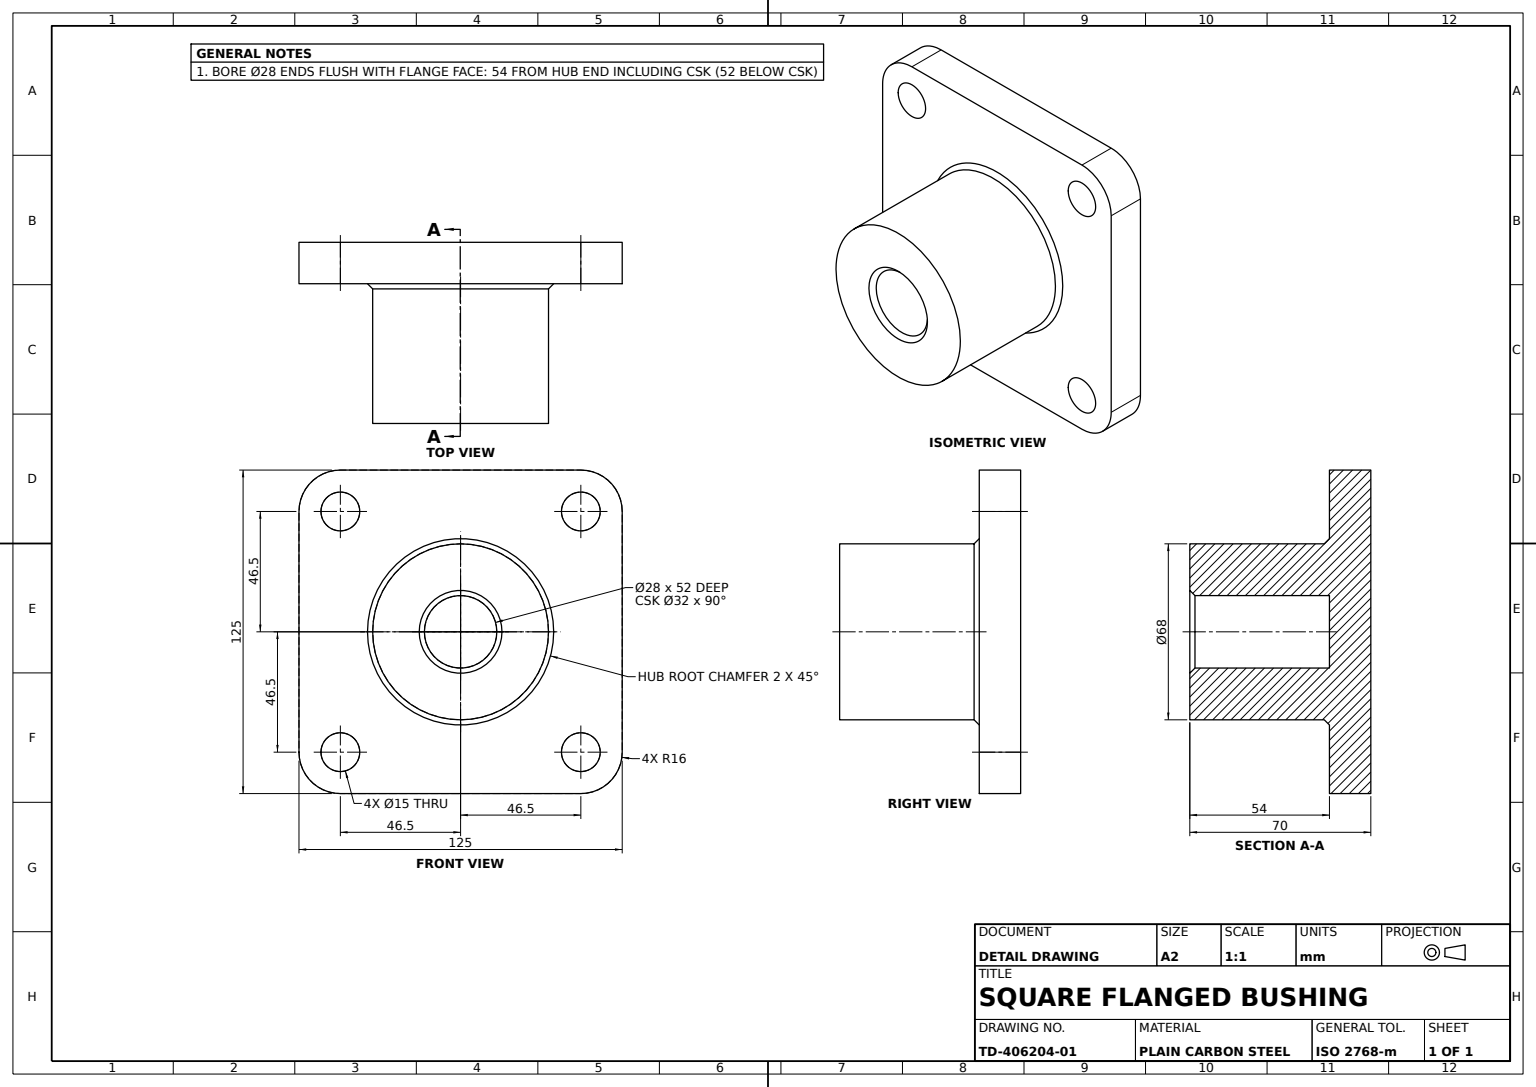
from build123d import *

# Parameters (mm, degrees)
FLANGE_PLATE_125X125X16_DEPTH = 16
BOLT_HOLES_SKETCH_R           = 7.5
BOLT_HOLES_4X_15_DEPTH        = 16
HUB_SKETCH_R                  = 34
HUB_68X54_DEPTH               = 54
HUB_CHAMFER_2X45_SIZE         = 2
BORE_SKETCH_R                 = 14
BORE_28_DEPTH                 = 54
BORE_CHAMFER_2X45_SIZE        = 2


with BuildPart() as part:
    # Flange Plate Sketch → Flange Plate 125x125x16 (new body)
    with BuildSketch(Plane.XY):
        with BuildLine():
            Line((16, 0), (109, 0))
            ThreePointArc((109, 0), (120.313708499, -4.686291501), (125, -16))
            Line((125, -16), (125, -109))
            ThreePointArc((125, -109), (120.313708499, -120.313708499), (109, -125))
            Line((109, -125), (16, -125))
            ThreePointArc((16, -125), (4.686291501, -120.313708499), (0, -109))
            Line((0, -109), (0, -16))
            ThreePointArc((0, -16), (4.686291501, -4.686291501), (16, 0))
        make_face()
    extrude(amount=FLANGE_PLATE_125X125X16_DEPTH)

    # Bolt Holes Sketch → Bolt Holes 4xØ15 (cut)
    with BuildSketch(Plane.XY.offset(16)):
        with Locations((16, -16)):
            Circle(BOLT_HOLES_SKETCH_R)
        with Locations((109, -16)):
            Circle(BOLT_HOLES_SKETCH_R)
        with Locations((109, -109)):
            Circle(BOLT_HOLES_SKETCH_R)
        with Locations((16, -109)):
            Circle(BOLT_HOLES_SKETCH_R)
    extrude(amount=-BOLT_HOLES_4X_15_DEPTH, mode=Mode.SUBTRACT)

    # Hub Sketch → Hub Ø68x54 (add)
    with BuildSketch(Plane.XY.offset(16)):
        with Locations((62.5, -62.5)):
            Circle(HUB_SKETCH_R)
    extrude(amount=HUB_68X54_DEPTH)

    # Hub Chamfer 2x45
    hub_chamfer_2x45_edges = [part.edges().sort_by_distance(p)[0] for p in [
        (28.5, -62.5, 16),
    ]]
    chamfer(hub_chamfer_2x45_edges, length=HUB_CHAMFER_2X45_SIZE)

    # Bore Sketch → Bore Ø28 (cut)
    with BuildSketch(Plane.XY.offset(70)):
        with Locations((62.5, -62.5)):
            Circle(BORE_SKETCH_R)
    extrude(amount=-BORE_28_DEPTH, mode=Mode.SUBTRACT)

    # Bore Chamfer 2x45
    bore_chamfer_2x45_edges = [part.edges().sort_by_distance(p)[0] for p in [
        (48.5, -62.5, 70),
    ]]
    chamfer(bore_chamfer_2x45_edges, length=BORE_CHAMFER_2X45_SIZE)


solid = part.part
